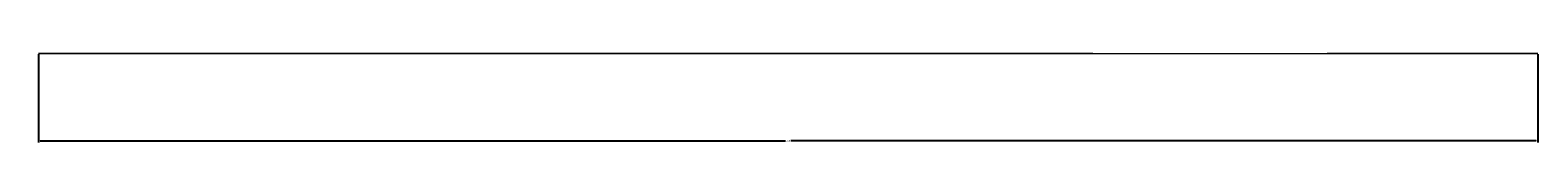
# Model space of a CAD drawing. Units: inches. Extents: x 1030 to 1191, y -9 to 0.
import ezdxf

# ---------------------------------------------------------------- set-up
doc = ezdxf.new("R2010")
doc.units = ezdxf.units.IN
doc.header["$MEASUREMENT"] = 0
doc.layers.add('M-CONS', color=7, linetype='Continuous', lineweight=18)
doc.layers.add('M-DIMS', color=2, linetype='Continuous', lineweight=18)
doc.styles.get("Standard").update_dxf_attribs({"font": 'arial.ttf'})
doc.dimstyles.get("Standard").update_dxf_attribs({"dimtxt": 0.18, "dimasz": 0.18, "dimexe": 0.18, "dimexo": 0.0625, "dimgap": 0.09, "dimtad": 0, "dimtih": 1, "dimtoh": 1, "dimdec": 4, "dimzin": 0, "dimdsep": 46, "dimtxsty": 'Standard', "dimcen": 0.09, "dimadec": 0, "dimazin": 0, "dimtfac": 1, "dimtdec": 4, "dimtofl": 0, "dimtmove": 0, "dimatfit": 3, "dimfxl": 1, "dimtolj": 1, "dimtzin": 0, "dimarcsym": 0})

# ---------------------------------------------------------------- blocks, each defined once
blk = doc.blocks.new('*D1')
at = {"layer": 'Defpoints', "color": 0, "transparency": 16777216}
for p in [(1030.63, 0), (1190.63, 0), (1190.63, -9.3)]:
    blk.add_point(p, dxfattribs=at)
at = {"layer": 'M-DIMS', "color": 0, "lineweight": -2, "transparency": 16777216}
for p, q in [((1030.63, -0.06), (1030.63, -9.48)), ((1190.63, -0.06), (1190.63, -9.48)), ((1030.81, -9.3), (1110.35, -9.3)), ((1190.45, -9.3), (1110.91, -9.3))]:
    blk.add_line(p, q, dxfattribs=at)
at = {"layer": 'M-DIMS', "color": 0, "transparency": 16777216}
for points in [[(1030.81, -9.27), (1030.81, -9.33), (1030.63, -9.3)], [(1190.45, -9.27), (1190.45, -9.33), (1190.63, -9.3)]]:
    blk.add_solid(points, dxfattribs=at)
at = {"layer": 'M-DIMS', "color": 0, "transparency": 16777216, "insert": (1110.63, -9.3), "char_height": 0.18, "attachment_point": 5}
blk.add_mtext('\\A1;160', dxfattribs=at)

msp = doc.modelspace()

# ---------------------------------------------------------------- linework, layer by layer
at = {"layer": 'M-CONS', "extrusion": (0, -1, 0)}
for p, q in [((1055.63, 0, 491.95), (1108.09, 0, 491.95)), ((1055.63, 0, 461.95), (1175.63, 0, 461.95)), ((1128.12, 0, 551.33), (1128.09, 0, 511.93)), ((1135.63, 0, 566.93), (1135.59, 0, 511.96)), ((1155.59, 0, 491.95), (1175.63, 0, 491.95))]:
    msp.add_line(p, q, dxfattribs=at)
for centre in [(1055.63, 476.95), (1095.63, 476.95), (1135.63, 476.95), (1175.63, 476.95)]:
    msp.add_circle(centre, 7.5, dxfattribs=at)
for centre, radius, start, end in [((1050.63, 529.45), 20, 150, 330), ((1115.58, 491.95), 95, 89.9633, 150), ((1050.63, 529.45), 12.5, 150, 330), ((1115.58, 491.95), 87.5, 89.9633, 150), ((1055.63, 476.95), 15, 90, 270), ((1115.58, 491.95), 62.5, 89.9559, 150), ((1115.58, 491.95), 55, 89.9499, 150), ((1108.09, 511.95), 20, 270, 359.9556), ((1115.63, 566.95), 20, 269.9633, 308.6378), ((1115.63, 566.95), 12.5, 269.9633, 90), ((1115.63, 566.95), 20, 359.9556, 90), ((1155.59, 511.95), 20, 179.9556, 270), ((1175.63, 476.95), 15, 270, 90)]:
    msp.add_arc(centre, radius, start, end, dxfattribs=at)

# ---------------------------------------------------------------- dimensions: what is measured, and where the dimension line sits
at = {"layer": 'M-DIMS'}
dim = msp.add_linear_dim(base=(1190.63, -9.3), p1=(1030.63, 0), p2=(1190.63, 0), dimstyle='Standard', override={"dimdec": 0, "dimlfac": 1, "dimrnd": 0, "dimzin": 0, "dimdsep": 46, "dimlunit": 2}, dxfattribs=at)
dim.commit()
dim.dimension.update_dxf_attribs({"geometry": '*D1', "text_midpoint": (1110.63, -9.3)})

doc.saveas('drawing.dxf')
